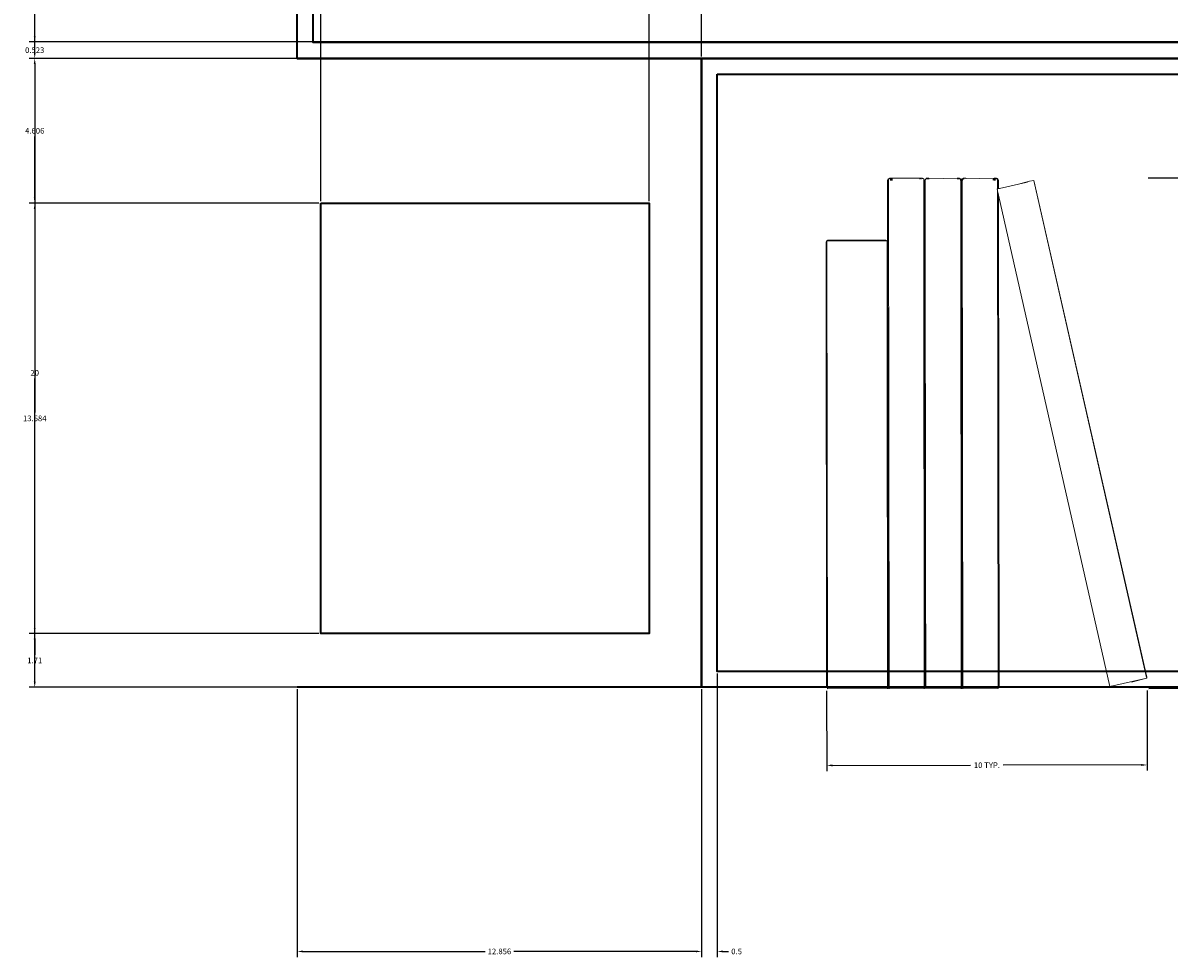
# Model space of a CAD drawing. Units: millimetres. Extents: x 446512 to 447461, y 70395 to 70610.
# Tile 1 of 39: x 446678 to 446714, y 70405 to 70435. Entities that reach past the tile are written whole.
import ezdxf

# ---------------------------------------------------------------- set-up
doc = ezdxf.new("R2010")
doc.units = ezdxf.units.MM
for name, color, linetype, lineweight in [('A-ANNO-DIMS', 2, 'Continuous', 18), ('A-CONS', 9, 'Continuous', 13), ('A-FURN', 7, 'Continuous', 35), ('A-FURN-DECO', 8, 'Continuous', 13)]:
    doc.layers.add(name, color=color, linetype=linetype, lineweight=lineweight)
doc.styles.get("Standard").update_dxf_attribs({"font": 'arial.ttf'})
doc.dimstyles.get("Standard").update_dxf_attribs({"dimtxt": 0.18, "dimasz": 0.18, "dimexe": 0.18, "dimexo": 0.0625, "dimgap": 0.09, "dimtad": 0, "dimtih": 1, "dimtoh": 1, "dimdec": 4, "dimzin": 0, "dimdsep": 46, "dimtxsty": 'Standard', "dimcen": 0.09, "dimadec": 0, "dimazin": 0, "dimtfac": 1, "dimtdec": 4, "dimtofl": 0, "dimtmove": 0, "dimatfit": 3, "dimfxl": 1, "dimtolj": 1, "dimtzin": 0, "dimarcsym": 0})

# ---------------------------------------------------------------- blocks, each defined once
blk = doc.blocks.new('DECO-VASE-C')
for p, q in [((1.958, 16.16), (1.977, 16.215)), ((1.977, 16.202), (1.958, 16.16)), ((1.958, 0.055), (1.958, 16.16)), ((1.977, 16.215), (1.982, 16.215)), ((1.977, 16.215), (1.977, 16.202)), ((1.982, 16.215), (1.977, 16.202)), ((1.977, 16.202), (1.977, 16.17)), ((1.982, 16.215), (1.989, 16.215)), ((1.989, 16.215), (1.988, 0)), ((1.989, 16.215), (1.997, 16.218)), ((1.997, 16.218), (2.035, 16.233)), ((2.016, 16.22), (1.997, 16.218)), ((1.997, 16.218), (2.009, 16.215)), ((2.019, 16.221), (2.016, 16.22)), ((3.07, 16.233), (2.035, 16.233)), ((2.054, 16.161), (2.053, 16.215)), ((2.058, 16.161), (2.058, 16.215)), ((2.088, 16.215), (2.094, 16.163)), ((2.088, 16.163), (2.088, 16.215)), ((2.088, 16.215), (2.09, 16.163)), ((2.106, 16.215), (2.11, 16.164)), ((2.969, 16.21), (2.969, 16.215)), ((2.976, 16.215), (2.969, 16.215)), ((2.999, 16.212), (2.999, 16.215)), ((3.004, 16.215), (3.004, 16.212)), ((3.034, 16.215), (3.004, 16.215)), ((3.058, 16.224), (3.11, 16.215)), ((3.07, 16.233), (3.111, 16.215)), ((3.111, 16.215), (3.11, 16.215)), ((3.114, 16.16), (3.111, 16.215)), ((3.115, 16.215), (3.111, 16.215)), ((3.114, 16.16), (3.113, 13.969)), ((3.114, 16.16), (3.115, 16.215)), ((3.133, 0.055), (3.114, 16.16)), ((3.133, 16.16), (3.177, 16.207)), ((3.152, 3.273), (3.133, 16.16)), ((3.133, 16.16), (3.153, 0.055)), ((3.152, 16.16), (3.177, 16.207)), ((3.152, 3.273), (3.152, 16.16)), ((3.177, 16.207), (3.184, 16.215)), ((3.184, 16.215), (3.19, 16.233)), ((3.184, 16.215), (3.23, 16.225)), ((3.27, 16.233), (3.19, 16.233)), ((3.221, 16.215), (3.263, 16.215)), ((3.263, 16.218), (3.263, 16.215)), ((3.263, 16.215), (3.281, 16.216)), ((3.281, 16.216), (3.27, 16.233)), ((3.281, 16.216), (4.174, 16.232)), ((4.171, 16.215), (4.179, 16.215)), ((4.176, 16.233), (4.174, 16.232)), ((4.178, 16.232), (4.176, 16.233)), ((4.178, 16.232), (4.232, 16.233)), ((4.179, 16.215), (4.179, 16.217)), ((4.209, 16.215), (4.179, 16.215)), ((4.209, 16.215), (4.196, 16.222)), ((4.214, 16.215), (4.209, 16.215)), ((4.212, 16.227), (4.224, 16.225)), ((4.224, 16.225), (4.214, 16.215)), ((4.232, 16.233), (4.224, 16.225)), ((4.224, 16.225), (4.249, 16.221)), ((4.232, 16.233), (4.249, 16.221)), ((4.249, 16.221), (4.258, 16.215)), ((4.249, 16.221), (4.285, 16.215)), ((4.283, 16.171), (4.258, 16.215)), ((4.279, 0), (4.29, 16.16)), ((4.283, 16.171), (4.285, 16.17)), ((4.29, 16.16), (4.283, 16.171)), ((4.309, 16.16), (4.285, 16.215)), ((4.285, 0), (4.309, 16.16)), ((4.29, 0), (4.309, 16.16)), ((4.309, 16.16), (4.327, 16.215)), ((4.332, 16.215), (4.309, 16.16)), ((4.309, 0.055), (4.309, 16.16)), ((4.309, 16.16), (4.327, 0.012)), ((4.327, 16.215), (4.332, 16.215)), ((4.327, 16.16), (4.36, 16.215)), ((4.331, 0.004), (4.327, 16.16)), ((4.332, 16.215), (4.363, 16.22)), ((4.36, 16.215), (4.332, 16.215)), ((4.36, 16.215), (4.363, 16.22)), ((4.396, 16.215), (4.36, 16.215)), ((4.363, 16.22), (4.37, 16.233)), ((4.363, 16.22), (4.384, 16.223)), ((4.439, 16.232), (4.37, 16.233)), ((4.438, 16.212), (4.438, 16.215)), ((4.442, 16.233), (4.439, 16.232)), ((4.439, 16.232), (4.444, 16.232)), ((4.442, 16.233), (4.444, 16.232)), ((4.442, 16.212), (4.442, 16.215)), ((4.444, 16.232), (5.319, 16.215)), ((4.469, 16.211), (4.47, 16.215)), ((5.319, 16.215), (5.317, 16.165)), ((5.319, 16.215), (5.322, 16.217)), ((5.322, 16.217), (5.351, 16.233)), ((5.322, 16.217), (5.35, 16.216)), ((5.35, 16.216), (5.348, 16.163)), ((5.351, 16.233), (5.35, 16.216)), ((5.35, 16.216), (5.354, 16.216)), ((5.351, 16.233), (5.354, 16.216)), ((5.383, 16.215), (5.351, 16.233)), ((5.351, 16.233), (5.422, 16.233)), ((5.351, 16.233), (5.398, 16.222)), ((5.403, 16.224), (5.351, 16.233)), ((5.354, 16.216), (5.352, 16.163)), ((5.354, 16.216), (5.355, 16.163)), ((5.354, 16.216), (5.383, 16.215)), ((5.383, 16.215), (5.386, 16.215)), ((5.383, 16.215), (5.384, 16.215)), ((5.384, 16.161), (5.384, 16.215)), ((5.384, 16.161), (5.386, 16.215)), ((5.384, 16.215), (5.386, 16.215)), ((5.386, 16.215), (5.433, 16.215)), ((5.386, 16.215), (5.388, 16.215)), ((5.388, 16.215), (5.398, 16.222)), ((5.398, 16.222), (5.4, 16.222)), ((5.4, 16.222), (5.403, 16.224)), ((5.4, 16.222), (5.433, 16.215)), ((5.405, 16.224), (5.403, 16.224)), ((5.405, 16.224), (5.422, 16.233)), ((5.449, 16.217), (5.405, 16.224)), ((5.449, 16.217), (5.422, 16.233)), ((5.433, 16.215), (5.449, 16.217)), ((5.453, 16.215), (5.449, 16.217)), ((5.453, 16.215), (5.453, 15.894)), ((5.465, 16.215), (5.453, 16.215)), ((5.465, 16.215), (5.484, 16.16)), ((5.465, 16.17), (5.465, 16.215)), ((5.484, 16.16), (5.484, 15.909)), ((5.516, 15.905), (6.127, 16.043)), ((6.127, 16.043), (6.476, 16.134)), ((6.127, 16.043), (6.409, 16.107)), ((6.614, 16.153), (6.476, 16.134)), ((6.615, 16.153), (6.614, 16.153)), ((6.614, 16.153), (10.177, 0.349)), ((10.188, 0.362), (6.615, 16.153)), ((5.442, 15.889), (5.453, 15.894)), ((5.442, 15.889), (5.454, 15.891)), ((5.453, 15.838), (5.442, 15.889)), ((5.453, 15.894), (5.484, 15.909)), ((5.453, 15.894), (5.454, 15.891)), ((5.453, 15.838), (5.453, 15.829)), ((5.453, 15.829), (5.454, 0)), ((5.485, 15.688), (5.453, 15.829)), ((5.516, 15.905), (5.454, 15.891)), ((5.492, 15.912), (5.484, 15.909)), ((5.484, 15.909), (5.484, 15.903)), ((5.485, 15.688), (5.484, 0.055)), ((5.485, 15.688), (8.218, 3.572)), ((5.492, 15.912), (5.516, 15.905)), ((0, 14.202), (0.014, 14.248)), ((0.014, 14.237), (0, 14.202)), ((0.014, 14.248), (0.018, 14.248)), ((0.014, 14.248), (0.014, 14.237)), ((0.018, 14.248), (0.014, 14.237)), ((0.014, 14.237), (0.014, 14.21)), ((0.018, 14.248), (0.023, 14.248)), ((0.023, 14.248), (0.029, 14.25)), ((0.023, 0), (0.023, 14.248)), ((0.029, 14.25), (0.06, 14.263)), ((0.029, 14.25), (0.066, 14.256)), ((0.074, 14.248), (0.029, 14.25)), ((0.06, 14.263), (0.104, 14.263)), ((0.066, 14.256), (0.06, 14.263)), ((0.066, 14.256), (0.104, 14.263)), ((0.074, 14.248), (0.066, 14.256)), ((0.074, 14.248), (0.094, 14.248)), ((0.094, 14.248), (0.104, 14.26)), ((0.101, 14.248), (0.094, 14.248)), ((0.101, 14.248), (0.104, 14.26)), ((0.101, 14.248), (0.105, 14.248)), ((0.107, 14.263), (0.104, 14.263)), ((0.104, 14.26), (0.104, 14.263)), ((0.105, 14.248), (0.104, 14.26)), ((0.104, 14.26), (0.129, 14.248)), ((0.129, 14.248), (0.105, 14.248)), ((0.129, 14.248), (0.107, 14.263)), ((0.107, 14.263), (1.898, 14.263)), ((1.839, 14.248), (0.129, 14.248)), ((1.842, 14.248), (1.839, 14.248)), ((1.857, 14.248), (1.842, 14.248)), ((1.857, 14.248), (1.898, 14.263)), ((1.857, 14.248), (1.88, 14.248)), ((1.88, 14.248), (1.884, 14.248)), ((1.883, 14.248), (1.88, 14.248)), ((1.884, 14.248), (1.883, 14.248)), ((1.898, 14.263), (1.884, 14.248)), ((1.884, 14.248), (1.89, 14.248)), ((1.89, 14.248), (1.94, 14.248)), ((1.898, 14.263), (1.94, 14.248)), ((1.944, 14.248), (1.94, 14.248)), ((1.943, 14.202), (1.94, 14.248)), ((1.943, 14.202), (1.944, 14.248)), ((0, 0.043), (0, 14.202)), ((1.943, 14.202), (1.941, 13.498)), ((1.958, 0.055), (1.943, 14.202)), ((3.113, 13.969), (3.104, 0)), ((3.113, 13.969), (3.133, 0.055)), ((1.941, 13.498), (1.944, 10.898)), ((1.944, 10.898), (1.935, 0)), ((1.944, 10.898), (1.958, 0.055)), ((1.945, 0.01), (1.944, 10.898)), ((8.218, 3.572), (9.007, 0.059)), ((9.01, 0.059), (8.218, 3.572)), ((0.023, 0), (5.454, 0)), ((10.183, 0.324), (9.01, 0.058)), ((10.06, 0.296), (9.693, 0.201)), ((10.06, 0.296), (10.181, 0.323)), ((10.183, 0.324), (10.177, 0.349)), ((10.177, 0.349), (10.181, 0.323)), ((10.183, 0.324), (10.181, 0.323)), ((10.188, 0.362), (10.183, 0.324))]:
    blk.add_line(p, q)
blk = doc.blocks.new('*D11')
at = {"layer": 'A-ANNO-DIMS', "color": 0, "lineweight": -2, "transparency": 16777216}
for p, q in [((446713.633, 70429.58), (446716.185, 70429.583)), ((446716.005, 70429.403), (446716.016, 70421.65)), ((446716.027, 70413.531), (446716.017, 70421.284)), ((446713.655, 70413.347), (446716.208, 70413.351))]:
    blk.add_line(p, q, dxfattribs=at)
at = {"layer": 'A-ANNO-DIMS', "color": 0, "transparency": 16777216}
for points in [[(446716.035, 70429.403), (446715.975, 70429.403), (446716.005, 70429.583)], [(446716.057, 70413.531), (446715.997, 70413.531), (446716.028, 70413.351)]]:
    blk.add_solid(points, dxfattribs=at)
at = {"layer": 'Defpoints', "color": 0, "transparency": 16777216}
for p in [(446713.57, 70429.58), (446716.005, 70429.583), (446713.593, 70413.347)]:
    blk.add_point(p, dxfattribs=at)
at = {"layer": 'A-ANNO-DIMS', "color": 0, "transparency": 16777216, "insert": (446716.016, 70421.467), "char_height": 0.18, "attachment_point": 5}
blk.add_mtext('\\A1;VASE C 16 TYP.', dxfattribs=at)
blk = doc.blocks.new('*D12')
at = {"layer": 'A-ANNO-DIMS', "color": 0, "lineweight": -2, "transparency": 16777216}
for p, q in [((446703.405, 70413.271), (446703.408, 70410.718)), ((446713.593, 70413.285), (446713.596, 70410.732)), ((446703.588, 70410.899), (446707.982, 70410.905)), ((446713.416, 70410.912), (446709.022, 70410.906))]:
    blk.add_line(p, q, dxfattribs=at)
at = {"layer": 'A-ANNO-DIMS', "color": 0, "transparency": 16777216}
for points in [[(446703.588, 70410.929), (446703.588, 70410.869), (446703.408, 70410.898)], [(446713.416, 70410.942), (446713.416, 70410.882), (446713.596, 70410.912)]]:
    blk.add_solid(points, dxfattribs=at)
at = {"layer": 'Defpoints', "color": 0, "transparency": 16777216}
for p in [(446703.405, 70413.333), (446713.593, 70413.347), (446713.596, 70410.912)]:
    blk.add_point(p, dxfattribs=at)
at = {"layer": 'A-ANNO-DIMS', "color": 0, "transparency": 16777216, "insert": (446708.502, 70410.905), "char_height": 0.18, "attachment_point": 5}
blk.add_mtext('\\A1;10 TYP.', dxfattribs=at)
blk = doc.blocks.new('*D18')
at = {"layer": 'A-ANNO-DIMS', "color": 0, "lineweight": -2, "transparency": 16777216}
for p, q in [((446686.51, 70433.382), (446678.043, 70433.382)), ((446678.223, 70433.202), (446678.223, 70423.563)), ((446678.223, 70413.562), (446678.223, 70423.2)), ((446749.161, 70413.382), (446678.043, 70413.382))]:
    blk.add_line(p, q, dxfattribs=at)
at = {"layer": 'A-ANNO-DIMS', "color": 0, "transparency": 16777216}
for points in [[(446678.193, 70433.202), (446678.253, 70433.202), (446678.223, 70433.382)], [(446678.193, 70413.562), (446678.253, 70413.562), (446678.223, 70413.382)]]:
    blk.add_solid(points, dxfattribs=at)
at = {"layer": 'Defpoints', "color": 0, "transparency": 16777216}
for p in [(446678.223, 70433.382), (446686.573, 70433.382), (446749.223, 70413.382)]:
    blk.add_point(p, dxfattribs=at)
at = {"layer": 'A-ANNO-DIMS', "color": 0, "transparency": 16777216, "insert": (446678.223, 70423.382), "char_height": 0.18, "attachment_point": 5}
blk.add_mtext('\\A1;20', dxfattribs=at)
blk = doc.blocks.new('*D19')
at = {"layer": 'A-ANNO-DIMS', "color": 0, "lineweight": -2, "transparency": 16777216}
for p, q in [((446686.51, 70453.382), (446678.043, 70453.382)), ((446678.223, 70453.202), (446678.223, 70443.563)), ((446678.223, 70433.562), (446678.223, 70443.2)), ((446686.51, 70433.382), (446678.043, 70433.382))]:
    blk.add_line(p, q, dxfattribs=at)
at = {"layer": 'A-ANNO-DIMS', "color": 0, "transparency": 16777216}
for points in [[(446678.193, 70453.202), (446678.253, 70453.202), (446678.223, 70453.382)], [(446678.193, 70433.562), (446678.253, 70433.562), (446678.223, 70433.382)]]:
    blk.add_solid(points, dxfattribs=at)
at = {"layer": 'Defpoints', "color": 0, "transparency": 16777216}
for p in [(446678.223, 70453.382), (446686.573, 70453.382), (446686.573, 70433.382)]:
    blk.add_point(p, dxfattribs=at)
at = {"layer": 'A-ANNO-DIMS', "color": 0, "transparency": 16777216, "insert": (446678.223, 70443.382), "char_height": 0.18, "attachment_point": 5}
blk.add_mtext('\\A1;20', dxfattribs=at)
blk = doc.blocks.new('*D28')
at = {"layer": 'A-ANNO-DIMS', "color": 0, "lineweight": -2, "transparency": 16777216}
for p, q in [((446678.223, 70434.085), (446678.223, 70434.265)), ((446731.164, 70433.905), (446678.043, 70433.905)), ((446728.946, 70433.382), (446678.043, 70433.382)), ((446678.223, 70433.202), (446678.223, 70433.022))]:
    blk.add_line(p, q, dxfattribs=at)
at = {"layer": 'A-ANNO-DIMS', "color": 0, "transparency": 16777216}
for points in [[(446678.193, 70434.085), (446678.253, 70434.085), (446678.223, 70433.905)], [(446678.193, 70433.202), (446678.253, 70433.202), (446678.223, 70433.382)]]:
    blk.add_solid(points, dxfattribs=at)
at = {"layer": 'Defpoints', "color": 0, "transparency": 16777216}
for p in [(446731.226, 70433.905), (446678.223, 70433.382), (446729.008, 70433.382)]:
    blk.add_point(p, dxfattribs=at)
at = {"layer": 'A-ANNO-DIMS', "color": 0, "transparency": 16777216, "insert": (446678.223, 70433.643), "char_height": 0.18, "attachment_point": 5}
blk.add_mtext('\\A1;0.523', dxfattribs=at)
blk = doc.blocks.new('*D37')
at = {"layer": 'A-ANNO-DIMS', "color": 0, "lineweight": -2, "transparency": 16777216}
for p, q in [((446686.392846, 70577.99492), (446686.212846, 70577.99492)), ((446686.572846, 70433.44405), (446686.572846, 70578.17492)), ((446687.323552, 70428.838404), (446687.323552, 70578.17492)), ((446687.503552, 70577.99492), (446687.683552, 70577.99492))]:
    blk.add_line(p, q, dxfattribs=at)
at = {"layer": 'A-ANNO-DIMS', "color": 0, "transparency": 16777216}
for points in [[(446686.392846, 70578.02492), (446686.392846, 70577.96492), (446686.572846, 70577.99492)], [(446687.503552, 70578.02492), (446687.503552, 70577.96492), (446687.323552, 70577.99492)]]:
    blk.add_solid(points, dxfattribs=at)
at = {"layer": 'Defpoints', "color": 0, "transparency": 16777216}
for p in [(446687.323552, 70577.99492), (446686.572846, 70433.38155), (446687.323552, 70428.775904)]:
    blk.add_point(p, dxfattribs=at)
at = {"layer": 'A-ANNO-DIMS', "color": 0, "transparency": 16777216, "insert": (446686.948199, 70577.99492), "char_height": 0.18, "attachment_point": 5}
blk.add_mtext('\\A1;0.75', dxfattribs=at)
blk = doc.blocks.new('*D38')
at = {"layer": 'A-ANNO-DIMS', "color": 0, "lineweight": -2, "transparency": 16777216}
for p, q in [((446687.323552, 70428.838404), (446687.323552, 70578.17492)), ((446687.503552, 70577.99492), (446692.090383, 70577.99492)), ((446697.585686, 70577.99492), (446692.998855, 70577.99492)), ((446697.765686, 70428.838404), (446697.765686, 70578.17492))]:
    blk.add_line(p, q, dxfattribs=at)
at = {"layer": 'A-ANNO-DIMS', "color": 0, "transparency": 16777216}
for points in [[(446687.503552, 70578.02492), (446687.503552, 70577.96492), (446687.323552, 70577.99492)], [(446697.585686, 70578.02492), (446697.585686, 70577.96492), (446697.765686, 70577.99492)]]:
    blk.add_solid(points, dxfattribs=at)
at = {"layer": 'Defpoints', "color": 0, "transparency": 16777216}
for p in [(446697.765686, 70577.99492), (446687.323552, 70428.775904), (446697.765686, 70428.775904)]:
    blk.add_point(p, dxfattribs=at)
at = {"layer": 'A-ANNO-DIMS', "color": 0, "transparency": 16777216, "insert": (446692.544619, 70577.99492), "char_height": 0.18, "attachment_point": 5}
blk.add_mtext('\\A1;10.442', dxfattribs=at)
blk = doc.blocks.new('*D39')
at = {"layer": 'A-ANNO-DIMS', "color": 0, "lineweight": -2, "transparency": 16777216}
for p, q in [((446697.766, 70428.838), (446697.766, 70578.175)), ((446697.946, 70577.995), (446698.212, 70577.995)), ((446699.249, 70577.995), (446698.982, 70577.995)), ((446699.429, 70433.444), (446699.429, 70578.175))]:
    blk.add_line(p, q, dxfattribs=at)
at = {"layer": 'A-ANNO-DIMS', "color": 0, "transparency": 16777216}
for points in [[(446697.946, 70578.025), (446697.946, 70577.965), (446697.766, 70577.995)], [(446699.249, 70578.025), (446699.249, 70577.965), (446699.429, 70577.995)]]:
    blk.add_solid(points, dxfattribs=at)
at = {"layer": 'Defpoints', "color": 0, "transparency": 16777216}
for p in [(446699.429, 70577.995), (446699.429, 70433.382), (446697.766, 70428.776)]:
    blk.add_point(p, dxfattribs=at)
at = {"layer": 'A-ANNO-DIMS', "color": 0, "transparency": 16777216, "insert": (446698.597, 70577.995), "char_height": 0.18, "attachment_point": 5}
blk.add_mtext('\\A1;1.663', dxfattribs=at)
blk = doc.blocks.new('*D40')
at = {"layer": 'A-ANNO-DIMS', "color": 0, "lineweight": -2, "transparency": 16777216}
for p, q in [((446686.573, 70413.319), (446686.573, 70404.803)), ((446699.429, 70413.319), (446699.429, 70404.803)), ((446686.753, 70404.983), (446692.546, 70404.983)), ((446699.249, 70404.983), (446693.456, 70404.983))]:
    blk.add_line(p, q, dxfattribs=at)
at = {"layer": 'A-ANNO-DIMS', "color": 0, "transparency": 16777216}
for points in [[(446686.753, 70405.013), (446686.753, 70404.953), (446686.573, 70404.983)], [(446699.249, 70405.013), (446699.249, 70404.953), (446699.429, 70404.983)]]:
    blk.add_solid(points, dxfattribs=at)
at = {"layer": 'Defpoints', "color": 0, "transparency": 16777216}
for p in [(446686.573, 70413.382), (446699.429, 70413.382), (446699.429, 70404.983)]:
    blk.add_point(p, dxfattribs=at)
at = {"layer": 'A-ANNO-DIMS', "color": 0, "transparency": 16777216, "insert": (446693.001, 70404.983), "char_height": 0.18, "attachment_point": 5}
blk.add_mtext('\\A1;12.856', dxfattribs=at)
blk = doc.blocks.new('*D41')
at = {"layer": 'A-ANNO-DIMS', "color": 0, "lineweight": -2, "transparency": 16777216}
for p, q in [((446699.929, 70413.819), (446699.929, 70404.803)), ((446699.429, 70413.319), (446699.429, 70404.803)), ((446699.249, 70404.983), (446699.069, 70404.983)), ((446700.109, 70404.983), (446700.289, 70404.983))]:
    blk.add_line(p, q, dxfattribs=at)
at = {"layer": 'A-ANNO-DIMS', "color": 0, "transparency": 16777216}
for points in [[(446699.249, 70405.013), (446699.249, 70404.953), (446699.429, 70404.983)], [(446700.109, 70405.013), (446700.109, 70404.953), (446699.929, 70404.983)]]:
    blk.add_solid(points, dxfattribs=at)
at = {"layer": 'Defpoints', "color": 0, "transparency": 16777216}
for p in [(446699.929, 70413.882), (446699.429, 70413.382), (446699.929, 70404.983)]:
    blk.add_point(p, dxfattribs=at)
at = {"layer": 'A-ANNO-DIMS', "color": 0, "transparency": 16777216, "insert": (446700.543, 70404.983), "char_height": 0.18, "attachment_point": 5}
blk.add_mtext('\\A1;0.5', dxfattribs=at)
blk = doc.blocks.new('*D42')
at = {"layer": 'A-ANNO-DIMS', "color": 0, "lineweight": -2, "transparency": 16777216}
for p, q in [((446687.261, 70415.092), (446678.043, 70415.092)), ((446678.223, 70414.912), (446678.223, 70414.417)), ((446678.223, 70413.562), (446678.223, 70414.057)), ((446686.51, 70413.382), (446678.043, 70413.382))]:
    blk.add_line(p, q, dxfattribs=at)
at = {"layer": 'A-ANNO-DIMS', "color": 0, "transparency": 16777216}
for points in [[(446678.193, 70414.912), (446678.253, 70414.912), (446678.223, 70415.092)], [(446678.193, 70413.562), (446678.253, 70413.562), (446678.223, 70413.382)]]:
    blk.add_solid(points, dxfattribs=at)
at = {"layer": 'Defpoints', "color": 0, "transparency": 16777216}
for p in [(446678.223, 70415.092), (446687.324, 70415.092), (446686.573, 70413.382)]:
    blk.add_point(p, dxfattribs=at)
at = {"layer": 'A-ANNO-DIMS', "color": 0, "transparency": 16777216, "insert": (446678.223, 70414.237), "char_height": 0.18, "attachment_point": 5}
blk.add_mtext('\\A1;1.71', dxfattribs=at)
blk = doc.blocks.new('*D43')
at = {"layer": 'A-ANNO-DIMS', "color": 0, "lineweight": -2, "transparency": 16777216}
for p, q in [((446687.261, 70428.776), (446678.043, 70428.776)), ((446678.223, 70428.596), (446678.223, 70422.116)), ((446678.223, 70415.272), (446678.223, 70421.752)), ((446687.261, 70415.092), (446678.043, 70415.092))]:
    blk.add_line(p, q, dxfattribs=at)
at = {"layer": 'A-ANNO-DIMS', "color": 0, "transparency": 16777216}
for points in [[(446678.193, 70428.596), (446678.253, 70428.596), (446678.223, 70428.776)], [(446678.193, 70415.272), (446678.253, 70415.272), (446678.223, 70415.092)]]:
    blk.add_solid(points, dxfattribs=at)
at = {"layer": 'Defpoints', "color": 0, "transparency": 16777216}
for p in [(446678.223, 70428.776), (446687.324, 70428.776), (446687.324, 70415.092)]:
    blk.add_point(p, dxfattribs=at)
at = {"layer": 'A-ANNO-DIMS', "color": 0, "transparency": 16777216, "insert": (446678.223, 70421.934), "char_height": 0.18, "attachment_point": 5}
blk.add_mtext('\\A1;13.684', dxfattribs=at)
blk = doc.blocks.new('*D44')
at = {"layer": 'A-ANNO-DIMS', "color": 0, "lineweight": -2, "transparency": 16777216}
for p, q in [((446686.51, 70433.382), (446678.043, 70433.382)), ((446678.223, 70433.202), (446678.223, 70431.261)), ((446678.223, 70428.956), (446678.223, 70430.897)), ((446687.261, 70428.776), (446678.043, 70428.776))]:
    blk.add_line(p, q, dxfattribs=at)
at = {"layer": 'A-ANNO-DIMS', "color": 0, "transparency": 16777216}
for points in [[(446678.193, 70433.202), (446678.253, 70433.202), (446678.223, 70433.382)], [(446678.193, 70428.956), (446678.253, 70428.956), (446678.223, 70428.776)]]:
    blk.add_solid(points, dxfattribs=at)
at = {"layer": 'Defpoints', "color": 0, "transparency": 16777216}
for p in [(446678.223, 70433.382), (446686.573, 70433.382), (446687.324, 70428.776)]:
    blk.add_point(p, dxfattribs=at)
at = {"layer": 'A-ANNO-DIMS', "color": 0, "transparency": 16777216, "insert": (446678.223, 70431.079), "char_height": 0.18, "attachment_point": 5}
blk.add_mtext('\\A1;4.606', dxfattribs=at)
blk = doc.blocks.new('*D45')
at = {"layer": 'A-ANNO-DIMS', "color": 0, "lineweight": -2, "transparency": 16777216}
for p, q in [((446787.57348, 70414.06155), (446787.57348, 70414.24155)), ((446699.991325, 70413.88155), (446787.75348, 70413.88155)), ((446699.491325, 70413.38155), (446787.75348, 70413.38155)), ((446787.57348, 70413.20155), (446787.57348, 70413.02155))]:
    blk.add_line(p, q, dxfattribs=at)
at = {"layer": 'A-ANNO-DIMS', "color": 0, "transparency": 16777216}
for points in [[(446787.54348, 70414.06155), (446787.60348, 70414.06155), (446787.57348, 70413.88155)], [(446787.54348, 70413.20155), (446787.60348, 70413.20155), (446787.57348, 70413.38155)]]:
    blk.add_solid(points, dxfattribs=at)
at = {"layer": 'Defpoints', "color": 0, "transparency": 16777216}
for p in [(446699.928825, 70413.88155), (446699.428825, 70413.38155), (446787.57348, 70413.38155)]:
    blk.add_point(p, dxfattribs=at)
at = {"layer": 'A-ANNO-DIMS', "color": 0, "transparency": 16777216, "insert": (446787.57348, 70413.63155), "char_height": 0.18, "attachment_point": 5}
blk.add_mtext('\\A1;0.5', dxfattribs=at)

msp = doc.modelspace()

# ---------------------------------------------------------------- linework, layer by layer
at = {"layer": 'A-CONS'}
msp.add_point((446686.5728, 70433.3815), dxfattribs=at)
at = {"layer": 'A-FURN'}
for p, q in [((446686.5728, 70433.3815), (446686.5728, 70453.3815)), ((446686.5728, 70433.3815), (446746.5728, 70433.3815)), ((446699.4288, 70433.3815), (446699.4288, 70413.3815)), ((446746.5728, 70413.3815), (446686.5728, 70413.3815))]:
    msp.add_line(p, q, dxfattribs=at)
for points in [[(446686.5728, 70453.3815), (446729.0084, 70453.3815), (446729.0084, 70433.3815), (446686.5728, 70433.3815)], [(446687.0728, 70452.8815), (446728.5084, 70452.8815), (446728.5084, 70433.8815), (446687.0728, 70433.8815)], [(446699.4288, 70433.3815), (446746.5728, 70433.3815), (446746.5728, 70413.3815), (446699.4288, 70413.3815)], [(446699.9288, 70432.8815), (446746.0728, 70432.8815), (446746.0728, 70413.8815), (446699.9288, 70413.8815)], [(446687.3236, 70428.7759), (446697.7657, 70428.7759), (446697.7657, 70415.0923), (446687.3236, 70415.0923)]]:
    msp.add_lwpolyline(points, close=True, dxfattribs=at)
at = {"layer": 'A-FURN-DECO'}
msp.add_line((446699.4288, 70415.3911), (446699.4288, 70430.815), dxfattribs=at)

# ---------------------------------------------------------------- block references
at = {"layer": 'A-FURN-DECO', "rotation": 0.0788209252993777}
msp.add_blockref('DECO-VASE-C', (446703.4049, 70413.333), dxfattribs=at)

# ---------------------------------------------------------------- dimensions: what is measured, and where the dimension line sits
at = {"layer": 'A-ANNO-DIMS'}
for base, p1, p2, override, picture, middle in [((446687.3236, 70577.9949), (446686.5728, 70433.3815), (446687.3236, 70428.7759), {"dimdec": 2, "dimlfac": 1, "dimrnd": 0, "dimzin": 0, "dimdsep": 46, "dimlunit": 2}, '*D37', (446686.9482, 70577.9949)), ((446697.7657, 70577.9949), (446687.3236, 70428.7759), (446697.7657, 70428.7759), {"dimdec": 3, "dimlfac": 1, "dimrnd": 0, "dimzin": 0, "dimdsep": 46, "dimlunit": 2}, '*D38', (446692.5446, 70577.9949)), ((446699.4288, 70577.9949), (446697.7657, 70428.7759), (446699.4288, 70433.3815), {"dimdec": 3, "dimlfac": 1, "dimrnd": 0, "dimzin": 0, "dimdsep": 46, "dimlunit": 2}, '*D39', (446698.5973, 70577.9949)), ((446699.9288, 70404.9832), (446699.4288, 70413.3815), (446699.9288, 70413.8815), {"dimdec": 1, "dimlfac": 1, "dimrnd": 0, "dimzin": 0, "dimdsep": 46, "dimlunit": 2}, '*D41', (446700.5434, 70404.9832)), ((446699.4288, 70404.9832), (446686.5728, 70413.3815), (446699.4288, 70413.3815), {"dimdec": 3, "dimlfac": 1, "dimrnd": 0, "dimzin": 0, "dimdsep": 46, "dimlunit": 2}, '*D40', (446693.0008, 70404.9832))]:
    dim = msp.add_linear_dim(base=base, p1=p1, p2=p2, dimstyle='Standard', override=override, dxfattribs=at)
    dim.commit()
    dim.dimension.update_dxf_attribs({"geometry": picture, "text_midpoint": middle})
for base, p1, p2, override, picture, middle in [((446678.2228, 70453.3815), (446686.5728, 70433.3815), (446686.5728, 70453.3815), {"dimdec": 0, "dimlfac": 1, "dimrnd": 0, "dimzin": 0, "dimdsep": 46, "dimlunit": 2}, '*D19', (446678.2228, 70443.3815)), ((446678.2228, 70433.3815), (446731.2264, 70433.9045), (446729.0084, 70433.3815), {"dimdec": 3, "dimlfac": 1, "dimrnd": 0, "dimzin": 0, "dimdsep": 46, "dimlunit": 2}, '*D28', (446678.2228, 70433.643)), ((446678.2228, 70433.3815), (446687.3236, 70428.7759), (446686.5728, 70433.3815), {"dimdec": 3, "dimlfac": 1, "dimrnd": 0, "dimzin": 0, "dimdsep": 46, "dimlunit": 2}, '*D44', (446678.2228, 70431.0787)), ((446678.2228, 70433.3815), (446749.2235, 70413.3815), (446686.5728, 70433.3815), {"dimdec": 0, "dimlfac": 1, "dimrnd": 0, "dimzin": 0, "dimdsep": 46, "dimlunit": 2}, '*D18', (446678.2228, 70423.3815)), ((446678.2228, 70428.7759), (446687.3236, 70415.0923), (446687.3236, 70428.7759), {"dimdec": 3, "dimlfac": 1, "dimrnd": 0, "dimzin": 0, "dimdsep": 46, "dimlunit": 2}, '*D43', (446678.2228, 70421.9341)), ((446678.2228, 70415.0923), (446686.5728, 70413.3815), (446687.3236, 70415.0923), {"dimdec": 2, "dimlfac": 1, "dimrnd": 0, "dimzin": 0, "dimdsep": 46, "dimlunit": 2}, '*D42', (446678.2228, 70414.2369)), ((446787.5735, 70413.3815), (446699.9288, 70413.8815), (446699.4288, 70413.3815), {"dimdec": 1, "dimlfac": 1, "dimrnd": 0, "dimzin": 0, "dimdsep": 46, "dimlunit": 2}, '*D45', (446787.5735, 70413.6315))]:
    dim = msp.add_linear_dim(base=base, p1=p1, p2=p2, angle=90, dimstyle='Standard', override=override, dxfattribs=at)
    dim.commit()
    dim.dimension.update_dxf_attribs({"geometry": picture, "text_midpoint": middle})
for base, p1, p2, angle, text, picture, middle in [((446716.0052, 70429.5831), (446713.5926, 70413.3472), (446713.5703, 70429.5798), 90.07882, 'VASE C <> TYP.', '*D11', (446716.0164, 70421.4668)), ((446713.596, 70410.9123), (446703.4047, 70413.3332), (446713.5926, 70413.3472), 0.07882, '<> TYP.', '*D12', (446708.502, 70410.9053))]:
    dim = msp.add_linear_dim(base=base, p1=p1, p2=p2, angle=angle, text=text, dimstyle='Standard', override={"dimdec": 0, "dimlfac": 1, "dimrnd": 0, "dimzin": 0, "dimdsep": 46, "dimlunit": 2}, dxfattribs=at)
    dim.commit()
    dim.dimension.update_dxf_attribs({"geometry": picture, "text_midpoint": middle})

doc.saveas('drawing.dxf')
